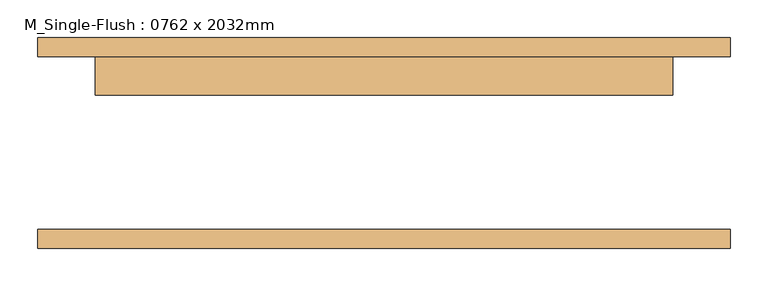
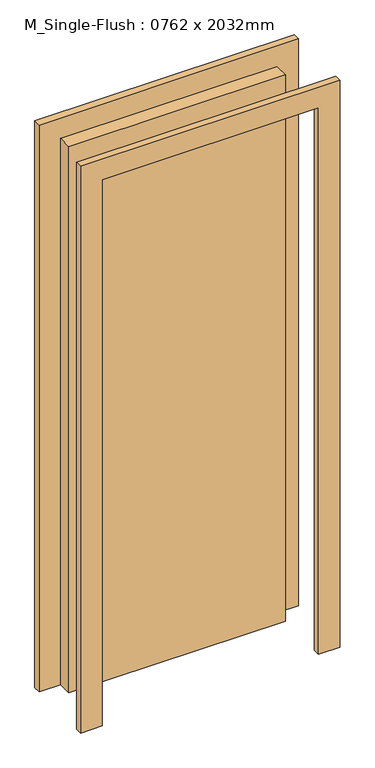
"""IFC4 building model written with IfcOpenShell, lengths in millimetres: door geometry, M_Single-Flush : 0762 x 2032mm."""

from ifc_helpers import new_model, si_unit, frame, origin, origin_with_axes, place, context, project, spatial, polyline, outline, extrude, source, transform, mapped, element, save


def m_single_flush_0762_x_2032mm_ddb9f746(model_context):
    return source(origin(), model_context, "Body", "SweptSolid", [
        extrude(outline(polyline([(2108.0, -457.0), (0.0, -457.0), (0.0, -381.0), (2032.0, -381.0), (2032.0, 381.0), (0.0, 381.0), (0.0, 457.0), (2108.0, 457.0), (2108.0, -457.0)])), frame((0.0, 114.3, 0.0), z_axis=(0.0, 1.0, 0.0), x_axis=(0.0, 0.0, 1.0)), (0.0, 0.0, 1.0), 25.0),
        extrude(outline(polyline([(2108.0, 457.0), (2108.0, -457.0), (0.0, -457.0), (0.0, -381.0), (2032.0, -381.0), (2032.0, 381.0), (0.0, 381.0), (0.0, 457.0), (2108.0, 457.0)])), frame((0.0, -139.3, 0.0), z_axis=(0.0, 1.0, 0.0), x_axis=(0.0, 0.0, 1.0)), (0.0, 0.0, 1.0), 25.0),
        extrude(outline(polyline([(381.0, 63.3), (-381.0, 63.3), (-381.0, 114.3), (381.0, 114.3), (381.0, 63.3)])), origin_with_axes(), (0.0, 0.0, 1.0), 2032.0),
    ])


if __name__ == "__main__":
    model = new_model("IFC4")
    model_context = context("Model", 3, world=origin())
    ifc_project = project(units=[si_unit("LENGTHUNIT", "METRE", prefix="MILLI")], contexts=[model_context])
    site = spatial("IfcSite", under=ifc_project)
    building = spatial("IfcBuilding", under=site)
    placement = place(None, origin())
    m_single_flush_0762_x_2032mm_shape = m_single_flush_0762_x_2032mm_ddb9f746(model_context)
    element("IfcDoor", 1, ObjectType="M_Single-Flush : 0762 x 2032mm", at=placement, inside=building, context=model_context, shape_type="MappedRepresentation", body=[
        mapped(m_single_flush_0762_x_2032mm_shape, transform((0.0, 0.0, 0.0), x_axis=(1.0, 0.0, 0.0), y_axis=(0.0, 1.0, 0.0), z_axis=(0.0, 0.0, 1.0))),
    ])
    save(model, "model.ifc")

# Revit data of these elements
# Type "M_Single-Flush : 0762 x 2032mm"
#   Type Mark = "19"
#   Thickness = 51 mm
#   Height = 2032 mm
#   Trim Projection Ext = 25 mm
#   Trim Projection Int = 25 mm
#   Trim Width = 76 mm
#   Width = 762 mm
#   Door Material = Door - Panel
#   Frame Material = Door - Frame
#   Function = (empty or 0)
#   Wall Closure = (empty or 0)
# Element 1 (IfcDoor, "M_Single-Flush : 0762 x 2032mm")
#   Materials on its faces: "Door - Frame", "Door - Panel"
# Materials
#   "Door - Panel": class "Wood", colour RGB 114 82 51, transparency 0
#   "Door - Frame": colour RGB 153 76 43, transparency 0
